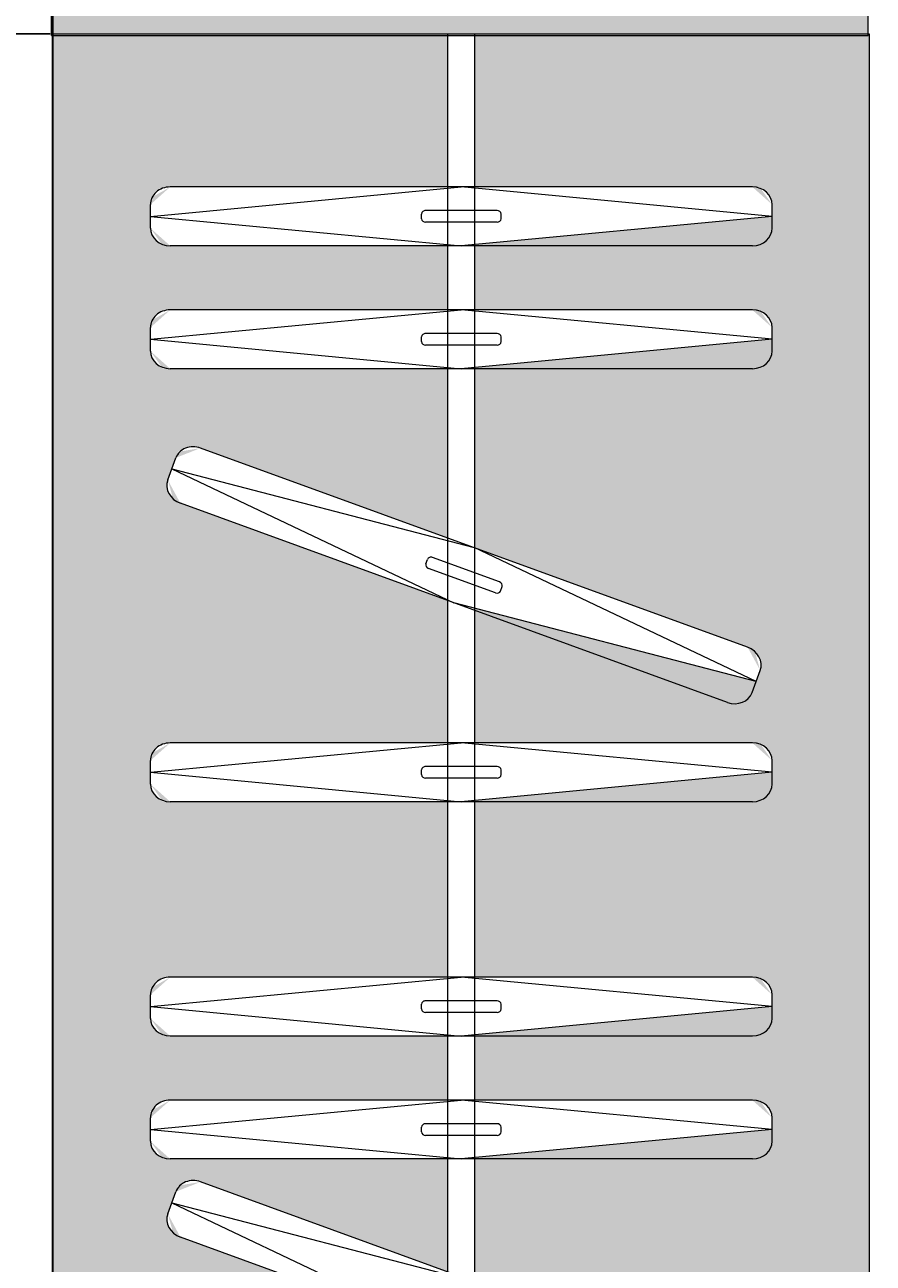
# Model space of a CAD drawing. Units: millimetres. Extents: x 27017497 to 27018854, y 7058029 to 7059154.
# Tile 70 of 91: x 27018319 to 27018341, y 7058174 to 7058207. Entities that reach past the tile are written whole.
import ezdxf

# ---------------------------------------------------------------- set-up
doc = ezdxf.new("R2010")
doc.units = ezdxf.units.MM
for name, color, linetype, lineweight in [('A-ANNO-DIMS', 2, 'Continuous', 18), ('A-FLOR-CASE', 8, 'Continuous', 20), ('A-FLOR-CASE-PATT', 44, 'Continuous', 13), ('A-WALL', 7, 'Continuous', 35)]:
    doc.layers.add(name, color=color, linetype=linetype, lineweight=lineweight)
doc.styles.get("Standard").update_dxf_attribs({"font": 'arial.ttf'})
doc.dimstyles.get("Standard").update_dxf_attribs({"dimtxt": 0.18, "dimasz": 0.18, "dimexe": 0.18, "dimexo": 0.0625, "dimgap": 0.09, "dimtad": 0, "dimtih": 1, "dimtoh": 1, "dimdec": 4, "dimzin": 0, "dimdsep": 46, "dimtxsty": 'Standard', "dimcen": 0.09, "dimadec": 0, "dimazin": 0, "dimtfac": 1, "dimtdec": 4, "dimtofl": 0, "dimtmove": 0, "dimatfit": 3, "dimfxl": 1, "dimtolj": 1, "dimtzin": 0, "dimarcsym": 0})

# ---------------------------------------------------------------- blocks, each defined once
blk = doc.blocks.new('WARDROBE-HANGING')
for p, q in [((0, 21.737), (65.212, 21.737)), ((0, 0), (0, 21.737)), ((4.862, 19.153), (4.08, 10.877)), ((5.175, 19.153), (4.549, 19.153)), ((4.862, 19.153), (5.645, 10.877)), ((8.135, 19.153), (7.353, 10.877)), ((8.448, 19.153), (7.822, 19.153)), ((8.135, 19.153), (8.918, 10.877)), ((19.663, 19.153), (18.88, 10.877)), ((19.976, 19.153), (19.35, 19.153)), ((19.663, 19.153), (20.445, 10.877)), ((25.9, 19.153), (25.118, 10.877)), ((26.213, 19.153), (25.587, 19.153)), ((25.9, 19.153), (26.683, 10.877)), ((29.173, 19.153), (28.391, 10.877)), ((29.486, 19.153), (28.86, 19.153)), ((29.173, 19.153), (29.956, 10.877)), ((17.54, 18.619), (16.952, 18.833)), ((4.08, 18.624), (4.08, 3.13)), ((5.645, 18.624), (5.645, 3.13)), ((7.353, 18.624), (7.353, 3.13)), ((8.918, 18.624), (8.918, 3.13)), ((16.33, 18.497), (11.031, 3.937)), ((17.246, 18.726), (13.68, 11.217)), ((17.246, 18.726), (15.151, 10.682)), ((18.88, 18.624), (18.88, 3.13)), ((20.445, 18.624), (20.445, 3.13)), ((25.118, 18.624), (25.118, 3.13)), ((26.683, 18.624), (26.683, 3.13)), ((28.391, 18.624), (28.391, 3.13)), ((29.956, 18.624), (29.956, 3.13)), ((35.867, 18.497), (30.567, 3.937)), ((17.801, 17.962), (12.501, 3.402)), ((37.337, 17.962), (32.038, 3.402)), ((4.925, 11.934), (4.8, 11.934)), ((8.198, 11.934), (8.073, 11.934)), ((14.594, 11.896), (13.943, 10.11)), ((14.836, 11.921), (14.718, 11.964)), ((19.725, 11.934), (19.6, 11.934)), ((25.963, 11.934), (25.838, 11.934)), ((29.236, 11.934), (29.111, 11.934)), ((4.706, 11.828), (4.706, 9.927)), ((5.019, 11.828), (5.019, 9.927)), ((7.979, 11.828), (7.979, 9.927)), ((8.292, 11.828), (8.292, 9.927)), ((14.888, 11.789), (14.237, 10.002)), ((19.506, 11.828), (19.506, 9.927)), ((19.819, 11.828), (19.819, 9.927)), ((25.744, 11.828), (25.744, 9.927)), ((26.057, 11.828), (26.057, 9.927)), ((29.017, 11.828), (29.017, 9.927)), ((29.33, 11.828), (29.33, 9.927)), ((0, 11.231), (65.212, 11.231)), ((11.585, 3.173), (13.68, 11.217)), ((31.122, 3.173), (33.217, 11.217)), ((4.862, 2.602), (4.08, 10.877)), ((4.862, 2.602), (5.645, 10.877)), ((8.135, 2.602), (7.353, 10.877)), ((8.135, 2.602), (8.918, 10.877)), ((11.585, 3.173), (15.151, 10.682)), ((19.663, 2.602), (18.88, 10.877)), ((19.663, 2.602), (20.445, 10.877)), ((25.9, 2.602), (25.118, 10.877)), ((25.9, 2.602), (26.683, 10.877)), ((29.173, 2.602), (28.391, 10.877)), ((29.173, 2.602), (29.956, 10.877)), ((31.122, 3.173), (34.688, 10.682)), ((0, 10.506), (65.212, 10.506)), ((14.113, 9.935), (13.995, 9.978)), ((4.925, 9.821), (4.8, 9.821)), ((8.198, 9.821), (8.073, 9.821)), ((19.725, 9.821), (19.6, 9.821)), ((25.963, 9.821), (25.838, 9.821)), ((29.236, 9.821), (29.111, 9.821)), ((11.879, 3.066), (11.291, 3.28)), ((31.416, 3.066), (30.828, 3.28)), ((5.175, 2.602), (4.549, 2.602)), ((8.448, 2.602), (7.822, 2.602)), ((19.976, 2.602), (19.35, 2.602)), ((26.213, 2.602), (25.587, 2.602)), ((29.486, 2.602), (28.86, 2.602)), ((0, 0), (65.212, 0))]:
    blk.add_line(p, q)
for centre, major_axis, start_param, end_param in [((4.549, 18.624), (0, 0.528), 0, 1.570796), ((5.175, 18.624), (0, 0.528), 4.712389, 6.283185), ((7.822, 18.624), (0, 0.528), 0, 1.570796), ((8.448, 18.624), (0, 0.528), 4.712389, 6.283185), ((19.35, 18.624), (0, 0.528), 0, 1.570796), ((19.976, 18.624), (0, 0.528), 4.712389, 6.283185), ((25.587, 18.624), (0, 0.528), 0, 1.570796), ((26.213, 18.624), (0, 0.528), 4.712389, 6.283185), ((28.86, 18.624), (0, 0.528), 0, 1.570796), ((29.486, 18.624), (0, 0.528), 4.712389, 6.283185), ((16.771, 18.336), (0.181, 0.496), 0, 1.570796), ((17.359, 18.122), (0.181, 0.496), -1.570796, 0), ((4.8, 11.828), (0, 0.106), 0, 1.570796), ((4.925, 11.828), (0, 0.106), -1.570796, 0), ((8.073, 11.828), (0, 0.106), 0, 1.570796), ((8.198, 11.828), (0, 0.106), -1.570796, 0), ((14.682, 11.864), (0.0361, 0.0993), 0, 1.570796), ((14.8, 11.821), (0.0361, 0.0993), 4.712389, 6.283185), ((19.6, 11.828), (0, 0.106), 0, 1.570796), ((19.725, 11.828), (0, 0.106), -1.570796, 0), ((25.838, 11.828), (0, 0.106), 0, 1.570796), ((25.963, 11.828), (0, 0.106), -1.570796, 0), ((29.111, 11.828), (0, 0.106), 0, 1.570796), ((29.236, 11.828), (0, 0.106), -1.570796, 0), ((4.8, 9.927), (0, 0.106), 1.570796, 3.141593), ((4.925, 9.927), (0, 0.106), 3.141593, 4.712389), ((8.073, 9.927), (0, 0.106), 1.570796, 3.141593), ((8.198, 9.927), (0, 0.106), 3.141593, 4.712389), ((14.032, 10.077), (0.0361, 0.0993), 1.570796, 3.141593), ((14.149, 10.035), (0.0361, 0.0993), 3.141593, 4.712389), ((19.6, 9.927), (0, 0.106), 1.570796, 3.141593), ((19.725, 9.927), (0, 0.106), 3.141593, 4.712389), ((25.838, 9.927), (0, 0.106), 1.570796, 3.141593), ((25.963, 9.927), (0, 0.106), 3.141593, 4.712389), ((29.111, 9.927), (0, 0.106), 1.570796, 3.141593), ((29.236, 9.927), (0, 0.106), 3.141593, 4.712389), ((11.472, 3.777), (0.181, 0.496), 1.570796, 3.141593), ((31.008, 3.777), (0.181, 0.496), 1.570796, 3.141593), ((12.06, 3.562), (0.181, 0.496), 3.141593, 4.712389), ((31.597, 3.562), (0.181, 0.496), 3.141593, 4.712389), ((4.549, 3.13), (0, 0.528), 1.570796, 3.141593), ((5.175, 3.13), (0, 0.528), 3.141593, 4.712389), ((7.822, 3.13), (0, 0.528), 1.570796, 3.141593), ((8.448, 3.13), (0, 0.528), 3.141593, 4.712389), ((19.35, 3.13), (0, 0.528), 1.570796, 3.141593), ((19.976, 3.13), (0, 0.528), 3.141593, 4.712389), ((25.587, 3.13), (0, 0.528), 1.570796, 3.141593), ((26.213, 3.13), (0, 0.528), 3.141593, 4.712389), ((28.86, 3.13), (0, 0.528), 1.570796, 3.141593), ((29.486, 3.13), (0, 0.528), 3.141593, 4.712389)]:
    blk.add_ellipse(centre, major_axis=major_axis, ratio=0.888892, start_param=start_param, end_param=end_param)
blk = doc.blocks.new('*D33')
at = {"layer": 'A-ANNO-DIMS', "color": 0, "lineweight": -2, "transparency": 16777216}
for p, q in [((27018319.543, 7058207.1), (27018309.644, 7058207.1)), ((27018309.824, 7058206.92), (27018309.824, 7058174.677)), ((27018309.824, 7058142.068), (27018309.824, 7058174.311)), ((27018319.543, 7058141.888), (27018309.644, 7058141.888))]:
    blk.add_line(p, q, dxfattribs=at)
at = {"layer": 'A-ANNO-DIMS', "color": 0, "transparency": 16777216}
for points in [[(27018309.794, 7058206.92), (27018309.854, 7058206.92), (27018309.824, 7058207.1)], [(27018309.794, 7058142.068), (27018309.854, 7058142.068), (27018309.824, 7058141.888)]]:
    blk.add_solid(points, dxfattribs=at)
at = {"layer": 'Defpoints', "color": 0, "transparency": 16777216}
for p in [(27018319.606, 7058207.1), (27018309.824, 7058141.888), (27018319.606, 7058141.888)]:
    blk.add_point(p, dxfattribs=at)
at = {"layer": 'A-ANNO-DIMS', "color": 0, "transparency": 16777216, "insert": (27018309.824, 7058174.494), "char_height": 0.18, "attachment_point": 5}
blk.add_mtext('\\A1;WARDROBE 65 TYP.', dxfattribs=at)
blk = doc.blocks.new('*D47')
at = {"layer": 'A-ANNO-DIMS', "color": 0, "lineweight": -2, "transparency": 16777216}
for p, q in [((27017561.166, 7058294.35), (27017561.166, 7058028.6)), ((27018790.606, 7058294.35), (27018790.606, 7058028.6)), ((27017561.346, 7058028.78), (27018175.431, 7058028.78)), ((27018790.426, 7058028.78), (27018176.341, 7058028.78))]:
    blk.add_line(p, q, dxfattribs=at)
at = {"layer": 'A-ANNO-DIMS', "color": 0, "transparency": 16777216}
for points in [[(27017561.346, 7058028.81), (27017561.346, 7058028.75), (27017561.166, 7058028.78)], [(27018790.426, 7058028.81), (27018790.426, 7058028.75), (27018790.606, 7058028.78)]]:
    blk.add_solid(points, dxfattribs=at)
at = {"layer": 'Defpoints', "color": 0, "transparency": 16777216}
for p in [(27017561.166, 7058294.412), (27018790.606, 7058294.412), (27018790.606, 7058028.78)]:
    blk.add_point(p, dxfattribs=at)
at = {"layer": 'A-ANNO-DIMS', "color": 0, "transparency": 16777216, "insert": (27018175.886, 7058028.78), "char_height": 0.18, "attachment_point": 5}
blk.add_mtext('\\A1;1229.4', dxfattribs=at)
blk = doc.blocks.new('*D48')
at = {"layer": 'A-ANNO-DIMS', "color": 0, "lineweight": -2, "transparency": 16777216}
for p, q in [((27018463.498, 7058622.912), (27017497.536, 7058622.912)), ((27017497.716, 7058622.732), (27017497.716, 7058357.753)), ((27017497.716, 7058092.41), (27017497.716, 7058357.389)), ((27018555.129, 7058092.23), (27017497.536, 7058092.23))]:
    blk.add_line(p, q, dxfattribs=at)
at = {"layer": 'A-ANNO-DIMS', "color": 0, "transparency": 16777216}
for points in [[(27017497.686, 7058622.732), (27017497.746, 7058622.732), (27017497.716, 7058622.912)], [(27017497.686, 7058092.41), (27017497.746, 7058092.41), (27017497.716, 7058092.23)]]:
    blk.add_solid(points, dxfattribs=at)
at = {"layer": 'Defpoints', "color": 0, "transparency": 16777216}
for p in [(27018463.561, 7058622.912), (27017497.716, 7058092.23), (27018555.192, 7058092.23)]:
    blk.add_point(p, dxfattribs=at)
at = {"layer": 'A-ANNO-DIMS', "color": 0, "transparency": 16777216, "insert": (27017497.716, 7058357.571), "char_height": 0.18, "attachment_point": 5}
blk.add_mtext('\\A1;530.7', dxfattribs=at)

msp = doc.modelspace()

# ---------------------------------------------------------------- hatches: boundary and pattern name
at = {"layer": 'A-FLOR-CASE-PATT'}
h = msp.add_hatch(color=256, dxfattribs=at)
h.dxf.hatch_style = 1
edge = h.paths.add_edge_path()
edge.add_line((27018341.343, 7058207.055), (27018330.837, 7058207.055))
edge.add_line((27018330.837, 7058207.055), (27018330.837, 7058203.02))
edge.add_line((27018330.837, 7058203.02), (27018338.424, 7058203.02))
edge.add_ellipse((27018338.23, 7058202.551), major_axis=(0.528, 0), ratio=0.888892, start_angle=0, end_angle=90, ccw=False)
edge.add_line((27018338.758, 7058202.551), (27018338.758, 7058202.238))
edge.add_line((27018338.758, 7058202.238), (27018330.837, 7058201.488))
edge.add_line((27018330.837, 7058201.488), (27018330.837, 7058199.747))
edge.add_line((27018330.837, 7058199.747), (27018338.424, 7058199.747))
edge.add_ellipse((27018338.23, 7058199.277), major_axis=(0.528, 0), ratio=0.888892, start_angle=0, end_angle=90, ccw=False)
edge.add_line((27018338.758, 7058199.277), (27018338.758, 7058198.964))
edge.add_line((27018338.758, 7058198.964), (27018330.837, 7058198.215))
edge.add_line((27018330.837, 7058198.215), (27018330.837, 7058193.415))
edge.add_line((27018330.837, 7058193.415), (27018338.284, 7058190.704))
edge.add_ellipse((27018337.942, 7058190.329), major_axis=(0.496, -0.181), ratio=0.888892, start_angle=0, end_angle=90, ccw=False)
edge.add_line((27018338.439, 7058190.148), (27018338.331, 7058189.854))
edge.add_line((27018338.331, 7058189.854), (27018330.837, 7058191.806))
edge.add_line((27018330.837, 7058191.806), (27018330.837, 7058188.22))
edge.add_line((27018330.837, 7058188.22), (27018338.424, 7058188.22))
edge.add_ellipse((27018338.23, 7058187.75), major_axis=(0.528, 0), ratio=0.888892, start_angle=0, end_angle=90, ccw=False)
edge.add_line((27018338.758, 7058187.75), (27018338.758, 7058187.437))
edge.add_line((27018338.758, 7058187.437), (27018330.837, 7058186.688))
edge.add_line((27018330.837, 7058186.688), (27018330.837, 7058181.982))
edge.add_line((27018330.837, 7058181.982), (27018338.424, 7058181.982))
edge.add_ellipse((27018338.23, 7058181.513), major_axis=(0.528, 0), ratio=0.888892, start_angle=0, end_angle=90, ccw=False)
edge.add_line((27018338.758, 7058181.513), (27018338.758, 7058181.199))
edge.add_line((27018338.758, 7058181.199), (27018330.837, 7058180.45))
edge.add_line((27018330.837, 7058180.45), (27018330.837, 7058178.709))
edge.add_line((27018330.837, 7058178.709), (27018338.424, 7058178.709))
edge.add_ellipse((27018338.23, 7058178.239), major_axis=(0.528, 0), ratio=0.888892, start_angle=0, end_angle=90, ccw=False)
edge.add_line((27018338.758, 7058178.239), (27018338.758, 7058177.926))
edge.add_line((27018338.758, 7058177.926), (27018330.837, 7058177.177))
edge.add_line((27018330.837, 7058177.177), (27018330.837, 7058173.878))
edge.add_line((27018330.837, 7058173.878), (27018338.284, 7058171.167))
edge.add_ellipse((27018337.942, 7058170.792), major_axis=(0.496, -0.181), ratio=0.888892, start_angle=0, end_angle=90, ccw=False)
edge.add_line((27018338.439, 7058170.611), (27018338.331, 7058170.317))
edge.add_line((27018338.331, 7058170.317), (27018330.837, 7058172.269))
edge.add_line((27018330.837, 7058172.269), (27018330.837, 7058168.293))
edge.add_line((27018330.837, 7058168.293), (27018338.424, 7058168.293))
edge.add_ellipse((27018338.23, 7058167.824), major_axis=(0.528, 0), ratio=0.888892, start_angle=0, end_angle=90, ccw=False)
edge.add_line((27018338.758, 7058167.824), (27018338.758, 7058167.511))
edge.add_line((27018338.758, 7058167.511), (27018330.837, 7058166.762))
edge.add_line((27018330.837, 7058166.762), (27018330.837, 7058160.389))
edge.add_line((27018330.837, 7058160.389), (27018338.424, 7058160.389))
edge.add_ellipse((27018338.23, 7058159.92), major_axis=(0.528, 0), ratio=0.888892, start_angle=0, end_angle=90, ccw=False)
edge.add_line((27018338.758, 7058159.92), (27018338.758, 7058159.607))
edge.add_line((27018338.758, 7058159.607), (27018330.837, 7058158.858))
edge.add_line((27018330.837, 7058158.858), (27018330.837, 7058157.116))
edge.add_line((27018330.837, 7058157.116), (27018338.424, 7058157.116))
edge.add_ellipse((27018338.23, 7058156.647), major_axis=(0.528, 0), ratio=0.888892, start_angle=0, end_angle=90, ccw=False)
edge.add_line((27018338.758, 7058156.647), (27018338.758, 7058156.334))
edge.add_line((27018338.758, 7058156.334), (27018330.837, 7058155.585))
edge.add_line((27018330.837, 7058155.585), (27018330.837, 7058150.784))
edge.add_line((27018330.837, 7058150.784), (27018338.284, 7058148.073))
edge.add_ellipse((27018337.942, 7058147.698), major_axis=(0.496, -0.181), ratio=0.888892, start_angle=0, end_angle=90, ccw=False)
edge.add_line((27018338.439, 7058147.517), (27018338.331, 7058147.223))
edge.add_line((27018338.331, 7058147.223), (27018330.837, 7058149.175))
edge.add_line((27018330.837, 7058149.175), (27018330.837, 7058145.589))
edge.add_line((27018330.837, 7058145.589), (27018338.424, 7058145.589))
edge.add_ellipse((27018338.23, 7058145.119), major_axis=(0.528, 0), ratio=0.888892, start_angle=0, end_angle=90, ccw=False)
edge.add_line((27018338.758, 7058145.119), (27018338.758, 7058144.806))
edge.add_line((27018338.758, 7058144.806), (27018330.837, 7058144.057))
edge.add_line((27018330.837, 7058144.057), (27018330.837, 7058141.912))
edge.add_line((27018330.837, 7058141.912), (27018341.343, 7058141.912))
edge.add_line((27018341.343, 7058141.912), (27018341.343, 7058207.055))
edge = h.paths.add_edge_path()
edge.add_line((27018330.112, 7058207.055), (27018319.606, 7058207.055))
edge.add_line((27018319.606, 7058207.055), (27018319.606, 7058141.912))
edge.add_line((27018319.606, 7058141.912), (27018330.112, 7058141.912))
edge.add_line((27018330.112, 7058141.912), (27018330.112, 7058144.024))
edge.add_line((27018330.112, 7058144.024), (27018322.543, 7058144.024))
edge.add_ellipse((27018322.736, 7058144.493), major_axis=(0.528, 0), ratio=0.888892, start_angle=180, end_angle=270, ccw=False)
edge.add_line((27018322.208, 7058144.493), (27018322.208, 7058145.291))
edge.add_ellipse((27018322.736, 7058145.119), major_axis=(0.528, 0), ratio=0.888892, start_angle=90, end_angle=180, ccw=False)
edge.add_line((27018322.736, 7058145.589), (27018330.112, 7058145.589))
edge.add_line((27018330.112, 7058145.589), (27018330.112, 7058149.382))
edge.add_line((27018330.112, 7058149.382), (27018322.826, 7058152.034))
edge.add_ellipse((27018323.168, 7058152.409), major_axis=(0.496, -0.181), ratio=0.888892, start_angle=180, end_angle=270, ccw=False)
edge.add_line((27018322.672, 7058152.59), (27018322.945, 7058153.34))
edge.add_ellipse((27018323.382, 7058152.997), major_axis=(0.496, -0.181), ratio=0.888892, start_angle=90, end_angle=180, ccw=False)
edge.add_line((27018323.543, 7058153.439), (27018330.112, 7058151.048))
edge.add_line((27018330.112, 7058151.048), (27018330.112, 7058155.551))
edge.add_line((27018330.112, 7058155.551), (27018322.543, 7058155.551))
edge.add_ellipse((27018322.736, 7058156.021), major_axis=(0.528, 0), ratio=0.888892, start_angle=180, end_angle=270, ccw=False)
edge.add_line((27018322.208, 7058156.021), (27018322.208, 7058156.819))
edge.add_ellipse((27018322.736, 7058156.647), major_axis=(0.528, 0), ratio=0.888892, start_angle=90, end_angle=180, ccw=False)
edge.add_line((27018322.736, 7058157.116), (27018330.112, 7058157.116))
edge.add_line((27018330.112, 7058157.116), (27018330.112, 7058158.824))
edge.add_line((27018330.112, 7058158.824), (27018322.543, 7058158.824))
edge.add_ellipse((27018322.736, 7058159.294), major_axis=(0.528, 0), ratio=0.888892, start_angle=180, end_angle=270, ccw=False)
edge.add_line((27018322.208, 7058159.294), (27018322.208, 7058160.092))
edge.add_ellipse((27018322.736, 7058159.92), major_axis=(0.528, 0), ratio=0.888892, start_angle=90, end_angle=180, ccw=False)
edge.add_line((27018322.736, 7058160.389), (27018330.112, 7058160.389))
edge.add_line((27018330.112, 7058160.389), (27018330.112, 7058166.728))
edge.add_line((27018330.112, 7058166.728), (27018322.543, 7058166.728))
edge.add_ellipse((27018322.736, 7058167.198), major_axis=(0.528, 0), ratio=0.888892, start_angle=180, end_angle=270, ccw=False)
edge.add_line((27018322.208, 7058167.198), (27018322.208, 7058167.996))
edge.add_ellipse((27018322.736, 7058167.824), major_axis=(0.528, 0), ratio=0.888892, start_angle=90, end_angle=180, ccw=False)
edge.add_line((27018322.736, 7058168.293), (27018330.112, 7058168.293))
edge.add_line((27018330.112, 7058168.293), (27018330.112, 7058172.476))
edge.add_line((27018330.112, 7058172.476), (27018322.826, 7058175.128))
edge.add_ellipse((27018323.168, 7058175.503), major_axis=(0.496, -0.181), ratio=0.888892, start_angle=180, end_angle=270, ccw=False)
edge.add_line((27018322.672, 7058175.684), (27018322.945, 7058176.433))
edge.add_ellipse((27018323.382, 7058176.091), major_axis=(0.496, -0.181), ratio=0.888892, start_angle=90, end_angle=180, ccw=False)
edge.add_line((27018323.543, 7058176.533), (27018330.112, 7058174.142))
edge.add_line((27018330.112, 7058174.142), (27018330.112, 7058177.144))
edge.add_line((27018330.112, 7058177.144), (27018322.543, 7058177.144))
edge.add_ellipse((27018322.736, 7058177.613), major_axis=(0.528, 0), ratio=0.888892, start_angle=180, end_angle=270, ccw=False)
edge.add_line((27018322.208, 7058177.613), (27018322.208, 7058178.411))
edge.add_ellipse((27018322.736, 7058178.239), major_axis=(0.528, 0), ratio=0.888892, start_angle=90, end_angle=180, ccw=False)
edge.add_line((27018322.736, 7058178.709), (27018330.112, 7058178.709))
edge.add_line((27018330.112, 7058178.709), (27018330.112, 7058180.417))
edge.add_line((27018330.112, 7058180.417), (27018322.543, 7058180.417))
edge.add_ellipse((27018322.736, 7058180.886), major_axis=(0.528, 0), ratio=0.888892, start_angle=180, end_angle=270, ccw=False)
edge.add_line((27018322.208, 7058180.886), (27018322.208, 7058181.684))
edge.add_ellipse((27018322.736, 7058181.513), major_axis=(0.528, 0), ratio=0.888892, start_angle=90, end_angle=180, ccw=False)
edge.add_line((27018322.736, 7058181.982), (27018330.112, 7058181.982))
edge.add_line((27018330.112, 7058181.982), (27018330.112, 7058186.655))
edge.add_line((27018330.112, 7058186.655), (27018322.543, 7058186.655))
edge.add_ellipse((27018322.736, 7058187.124), major_axis=(0.528, 0), ratio=0.888892, start_angle=180, end_angle=270, ccw=False)
edge.add_line((27018322.208, 7058187.124), (27018322.208, 7058187.922))
edge.add_ellipse((27018322.736, 7058187.75), major_axis=(0.528, 0), ratio=0.888892, start_angle=90, end_angle=180, ccw=False)
edge.add_line((27018322.736, 7058188.22), (27018330.112, 7058188.22))
edge.add_line((27018330.112, 7058188.22), (27018330.112, 7058192.013))
edge.add_line((27018330.112, 7058192.013), (27018322.826, 7058194.665))
edge.add_ellipse((27018323.168, 7058195.04), major_axis=(0.496, -0.181), ratio=0.888892, start_angle=180, end_angle=270, ccw=False)
edge.add_line((27018322.672, 7058195.22), (27018322.945, 7058195.97))
edge.add_ellipse((27018323.382, 7058195.628), major_axis=(0.496, -0.181), ratio=0.888892, start_angle=90, end_angle=180, ccw=False)
edge.add_line((27018323.543, 7058196.069), (27018330.112, 7058193.678))
edge.add_line((27018330.112, 7058193.678), (27018330.112, 7058198.182))
edge.add_line((27018330.112, 7058198.182), (27018322.543, 7058198.182))
edge.add_ellipse((27018322.736, 7058198.651), major_axis=(0.528, 0), ratio=0.888892, start_angle=180, end_angle=270, ccw=False)
edge.add_line((27018322.208, 7058198.651), (27018322.208, 7058199.449))
edge.add_ellipse((27018322.736, 7058199.277), major_axis=(0.528, 0), ratio=0.888892, start_angle=90, end_angle=180, ccw=False)
edge.add_line((27018322.736, 7058199.747), (27018330.112, 7058199.747))
edge.add_line((27018330.112, 7058199.747), (27018330.112, 7058201.455))
edge.add_line((27018330.112, 7058201.455), (27018322.543, 7058201.455))
edge.add_ellipse((27018322.736, 7058201.924), major_axis=(0.528, 0), ratio=0.888892, start_angle=180, end_angle=270, ccw=False)
edge.add_line((27018322.208, 7058201.924), (27018322.208, 7058202.722))
edge.add_ellipse((27018322.736, 7058202.551), major_axis=(0.528, 0), ratio=0.888892, start_angle=90, end_angle=180, ccw=False)
edge.add_line((27018322.736, 7058203.02), (27018330.112, 7058203.02))
edge.add_line((27018330.112, 7058203.02), (27018330.112, 7058207.055))
h.paths.add_polyline_path([(27018341.31, 7058294.412), (27018319.606, 7058294.412), (27018319.606, 7058207.1), (27018341.31, 7058207.1)])
h.paths.add_polyline_path([(27018354.358, 7058255.592), (27018354.358, 7058256.057, -0.414214), (27018354.869, 7058256.569), (27018346.477, 7058256.569, -0.414214), (27018345.197, 7058257.848), (27018345.197, 7058259.128, -0.414214), (27018346.477, 7058260.407), (27018343.868, 7058260.407, 0.290979), (27018341.551, 7058258.934), (27018341.551, 7058242.534, 0.290979), (27018343.868, 7058241.06), (27018346.477, 7058241.06, -0.414214), (27018345.197, 7058242.34), (27018345.197, 7058243.619, -0.414214), (27018346.477, 7058244.899), (27018353.078, 7058244.899, 0.414214), (27018354.358, 7058246.178)])
h.paths.add_polyline_path([(27018356.917, 7058260.407), (27018346.477, 7058260.407, 0.414214), (27018345.197, 7058259.128), (27018345.197, 7058257.848, 0.414214), (27018346.477, 7058256.569), (27018355.637, 7058256.569), (27018355.637, 7058244.899), (27018346.477, 7058244.899, 0.414214), (27018345.197, 7058243.619), (27018345.197, 7058242.34, 0.414214), (27018346.477, 7058241.06), (27018356.917, 7058241.06, 0.414214), (27018359.476, 7058243.619), (27018359.476, 7058257.848, 0.414214)])
h.paths.add_polyline_path([(27018355.637, 7058252.362), (27018355.637, 7058256.057, 0.490314), (27018354.997, 7058256.553, 0.490314), (27018354.358, 7058256.057), (27018354.358, 7058255.592), (27018354.358, 7058245.411, 0.490314), (27018354.997, 7058244.915, 0.490314), (27018355.637, 7058245.411)], flags=17)

# ---------------------------------------------------------------- linework, layer by layer
at = {"layer": 'A-FLOR-CASE'}
for p, q in [((27018341.31, 7058207.055), (27018341.31, 7058294.412)), ((27018319.573, 7058207.055), (27018319.573, 7058251.237)), ((27018319.573, 7058207.055), (27018336.597, 7058207.055)), ((27018319.573, 7058207.055), (27018341.31, 7058207.055))]:
    msp.add_line(p, q, dxfattribs=at)
at = {"layer": 'A-WALL'}
msp.add_line((27018319.606, 7058386.803), (27018319.606, 7058141.912), dxfattribs=at)

# ---------------------------------------------------------------- block references
at = {"layer": 'A-FLOR-CASE', "rotation": 270}
msp.add_blockref('WARDROBE-HANGING', (27018319.606, 7058207.1), dxfattribs=at)

# ---------------------------------------------------------------- dimensions: what is measured, and where the dimension line sits
at = {"layer": 'A-ANNO-DIMS'}
dim = msp.add_linear_dim(base=(27017497.716, 7058092.23), p1=(27018463.561, 7058622.912), p2=(27018555.192, 7058092.23), angle=90, dimstyle='Standard', override={"dimdec": 1, "dimlfac": 1, "dimrnd": 0, "dimzin": 0, "dimdsep": 46, "dimlunit": 2}, dxfattribs=at)
dim.commit()
dim.dimension.update_dxf_attribs({"geometry": '*D48', "text_midpoint": (27017497.716, 7058357.571)})
dim = msp.add_linear_dim(base=(27018790.606, 7058028.78), p1=(27017561.166, 7058294.412), p2=(27018790.606, 7058294.412), dimstyle='Standard', override={"dimdec": 1, "dimlfac": 1, "dimrnd": 0, "dimzin": 0, "dimdsep": 46, "dimlunit": 2}, dxfattribs=at)
dim.commit()
dim.dimension.update_dxf_attribs({"geometry": '*D47', "text_midpoint": (27018175.886, 7058028.78)})
dim = msp.add_linear_dim(base=(27018309.824, 7058141.888), p1=(27018319.606, 7058207.1), p2=(27018319.606, 7058141.888), angle=270, text='WARDROBE <> TYP.', dimstyle='Standard', override={"dimdec": 0, "dimlfac": 1, "dimrnd": 0, "dimzin": 0, "dimdsep": 46, "dimlunit": 2}, dxfattribs=at)
dim.commit()
dim.dimension.update_dxf_attribs({"geometry": '*D33', "text_midpoint": (27018309.824, 7058174.494)})

doc.saveas('drawing.dxf')
